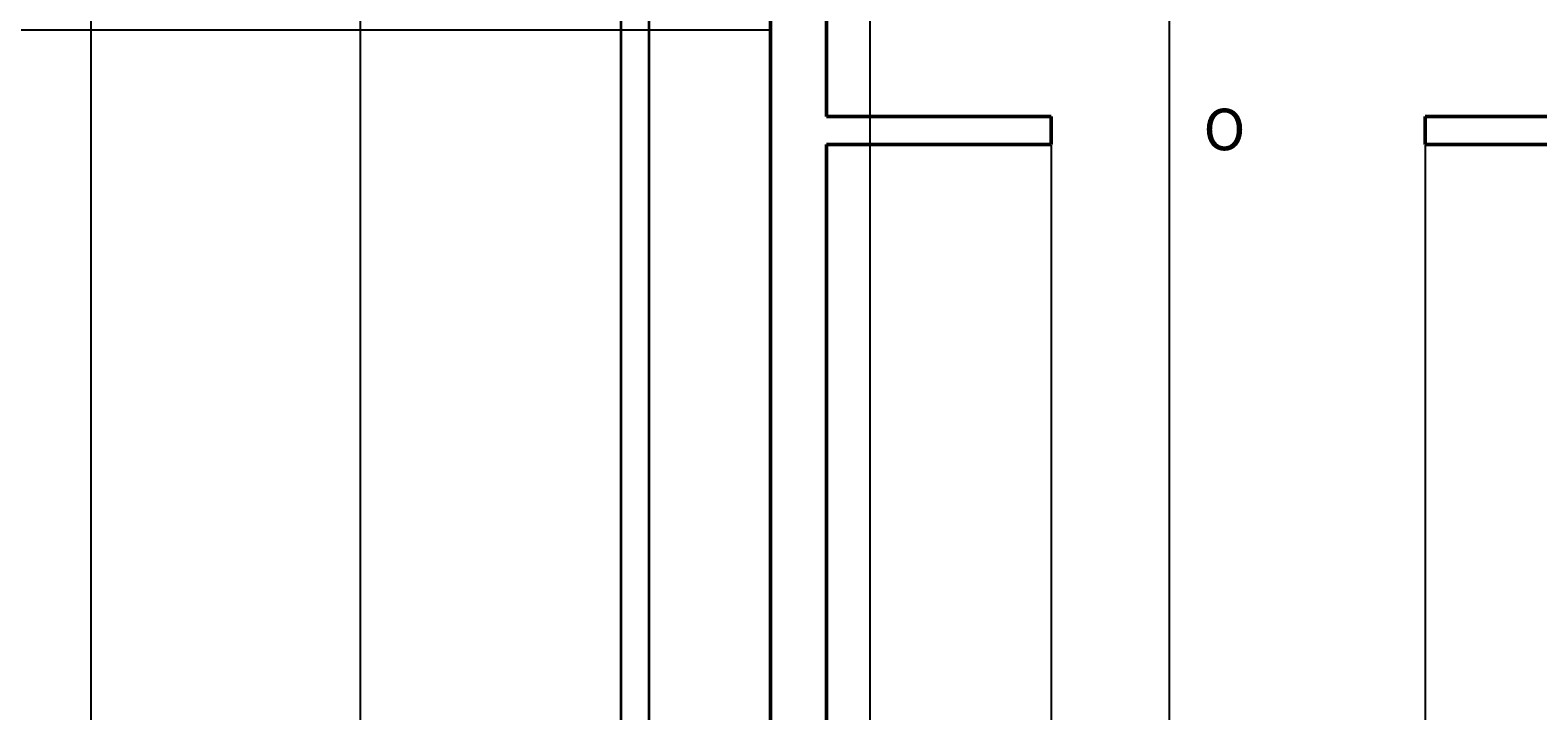
# Model space of a CAD drawing. Units: inches. Extents: x 338 to 1188, y -996 to 127.
# Tile 6 of 15: x 478 to 720, y -240 to -131. Entities that reach past the tile are written whole.
import ezdxf

# ---------------------------------------------------------------- set-up
doc = ezdxf.new("R2010")
doc.units = ezdxf.units.IN
doc.header["$MEASUREMENT"] = 0
for name, color, linetype, lineweight in [('A-ANNO-DIMS', 5, 'Continuous', 18), ('A-ANNO-TEXT', 7, 'Continuous', 18), ('C-PROP', 1, 'Continuous', 35), ('wall', 1, 'Continuous', 50)]:
    doc.layers.add(name, color=color, linetype=linetype, lineweight=lineweight)
doc.styles.get("Standard").update_dxf_attribs({"font": 'arial.ttf'})
doc.dimstyles.get("Standard").update_dxf_attribs({"dimtxt": 0.18, "dimasz": 0.18, "dimexe": 0.18, "dimexo": 0.0625, "dimgap": 0.09, "dimtad": 0, "dimtih": 1, "dimtoh": 1, "dimdec": 1, "dimzin": 0, "dimdsep": 46, "dimlunit": 4, "dimtxsty": 'Standard', "dimcen": 0.09, "dimadec": 0, "dimazin": 0, "dimtfac": 1, "dimtdec": 1, "dimtofl": 0, "dimtmove": 0, "dimatfit": 3, "dimfxl": 1, "dimtolj": 1, "dimtzin": 0, "dimarcsym": 0})

# ---------------------------------------------------------------- blocks, each defined once
blk = doc.blocks.new('_ArchTick')
at = {"color": 0, "linetype": 'ByBlock', "const_width": 0.15}
blk.add_lwpolyline([(-0.5, -0.5), (0.5, 0.5)], dxfattribs=at)
blk = doc.blocks.new('*D6')
at = {"layer": 'A-ANNO-DIMS', "color": 0, "lineweight": -2, "transparency": 16777216}
for p, q in [((531.19, -15.73), (531.19, -304.1)), ((531.19, -615.73), (531.19, -327.37))]:
    blk.add_line(p, q, dxfattribs=at)
at = {"layer": 'Defpoints', "color": 0, "transparency": 16777216}
for p in [(596.96, -15.73), (531.19, -615.73), (596.96, -615.73)]:
    blk.add_point(p, dxfattribs=at)
at = {"layer": 'A-ANNO-DIMS', "color": 0, "lineweight": -2, "transparency": 16777216, "xscale": 10, "yscale": 10, "zscale": 10}
for p, rotation in [((531.19, -15.73), 90), ((531.19, -615.73), 270)]:
    blk.add_blockref('_ArchTick', p, dxfattribs=dict(at, rotation=rotation))
at = {"layer": 'A-ANNO-DIMS', "color": 0, "transparency": 16777216, "insert": (531.19, -315.73), "char_height": 9, "attachment_point": 5, "rotation": 90}
blk.add_mtext("\\A1;50'", dxfattribs=at)
blk = doc.blocks.new('*D7')
at = {"layer": 'A-ANNO-DIMS', "color": 0, "lineweight": -2, "transparency": 16777216}
for p, q in [((488.01, 8.27), (488.01, -388.07)), ((488.01, -807.73), (488.01, -411.39))]:
    blk.add_line(p, q, dxfattribs=at)
at = {"layer": 'Defpoints', "color": 0, "transparency": 16777216}
for p in [(572.96, 8.27), (488.01, -807.73), (572.96, -807.73)]:
    blk.add_point(p, dxfattribs=at)
at = {"layer": 'A-ANNO-DIMS', "color": 0, "lineweight": -2, "transparency": 16777216, "xscale": 10, "yscale": 10, "zscale": 10}
for p, rotation in [((488.01, 8.27), 90), ((488.01, -807.73), 270)]:
    blk.add_blockref('_ArchTick', p, dxfattribs=dict(at, rotation=rotation))
at = {"layer": 'A-ANNO-DIMS', "color": 0, "transparency": 16777216, "insert": (488.01, -399.73), "char_height": 9, "attachment_point": 5, "rotation": 90}
blk.add_mtext("\\A1;68'", dxfattribs=at)
blk = doc.blocks.new('*D31')
at = {"layer": 'A-ANNO-DIMS', "color": 0, "lineweight": -2, "transparency": 16777216}
for p, q in [((641.96, -149.3), (641.96, -968.86)), ((701.96, -149.3), (701.96, -968.86)), ((642.14, -968.68), (671.63, -968.68)), ((701.78, -968.68), (672.29, -968.68))]:
    blk.add_line(p, q, dxfattribs=at)
at = {"layer": 'A-ANNO-DIMS', "color": 0, "transparency": 16777216}
for points in [[(642.14, -968.65), (642.14, -968.71), (641.96, -968.68)], [(701.78, -968.65), (701.78, -968.71), (701.96, -968.68)]]:
    blk.add_solid(points, dxfattribs=at)
at = {"layer": 'Defpoints', "color": 0, "transparency": 16777216}
for p in [(641.96, -149.23), (701.96, -149.23), (701.96, -968.68)]:
    blk.add_point(p, dxfattribs=at)
at = {"layer": 'A-ANNO-DIMS', "color": 0, "transparency": 16777216, "insert": (671.96, -968.68), "char_height": 0.18, "attachment_point": 5}
blk.add_mtext('\\A1;5\'-0"', dxfattribs=at)
blk = doc.blocks.new('*D34')
at = {"layer": 'A-ANNO-DIMS', "color": 0, "lineweight": -2, "transparency": 16777216}
for p, q in [((612.96, -615.67), (612.96, 67.25)), ((613.14, 67.07), (636.63, 67.07)), ((660.78, 67.07), (637.3, 67.07)), ((660.96, -615.67), (660.96, 67.25))]:
    blk.add_line(p, q, dxfattribs=at)
at = {"layer": 'A-ANNO-DIMS', "color": 0, "transparency": 16777216}
for points in [[(613.14, 67.1), (613.14, 67.04), (612.96, 67.07)], [(660.78, 67.1), (660.78, 67.04), (660.96, 67.07)]]:
    blk.add_solid(points, dxfattribs=at)
at = {"layer": 'Defpoints', "color": 0, "transparency": 16777216}
for p in [(660.96, 67.07), (612.96, -615.73), (660.96, -615.73)]:
    blk.add_point(p, dxfattribs=at)
at = {"layer": 'A-ANNO-DIMS', "color": 0, "transparency": 16777216, "insert": (636.96, 67.07), "char_height": 0.18, "attachment_point": 5}
blk.add_mtext('\\A1;4\'-0"', dxfattribs=at)
blk = doc.blocks.new('*D48')
at = {"layer": 'A-ANNO-DIMS', "color": 0, "lineweight": -2, "transparency": 16777216}
for p, q in [((596.96, -615.67), (596.96, 67.25)), ((597.14, 67.07), (604.64, 67.07)), ((612.78, 67.07), (605.28, 67.07)), ((612.96, -615.67), (612.96, 67.25))]:
    blk.add_line(p, q, dxfattribs=at)
at = {"layer": 'A-ANNO-DIMS', "color": 0, "transparency": 16777216}
for points in [[(597.14, 67.1), (597.14, 67.04), (596.96, 67.07)], [(612.78, 67.1), (612.78, 67.04), (612.96, 67.07)]]:
    blk.add_solid(points, dxfattribs=at)
at = {"layer": 'Defpoints', "color": 0, "transparency": 16777216}
for p in [(612.96, 67.07), (596.96, -615.73), (612.96, -615.73)]:
    blk.add_point(p, dxfattribs=at)
at = {"layer": 'A-ANNO-DIMS', "color": 0, "transparency": 16777216, "insert": (604.96, 67.07), "char_height": 0.18, "attachment_point": 5}
blk.add_mtext('\\A1;1\'-4"', dxfattribs=at)
blk = doc.blocks.new('*D51')
at = {"layer": 'A-ANNO-DIMS', "color": 0, "lineweight": -2, "transparency": 16777216}
for p, q in [((596.9, -130.89), (337.66, -130.89)), ((337.84, -131.07), (337.84, -187.13)), ((337.84, -243.55), (337.84, -187.49)), ((596.9, -243.73), (337.66, -243.73))]:
    blk.add_line(p, q, dxfattribs=at)
at = {"layer": 'A-ANNO-DIMS', "color": 0, "transparency": 16777216}
for points in [[(337.81, -131.07), (337.87, -131.07), (337.84, -130.89)], [(337.81, -243.55), (337.87, -243.55), (337.84, -243.73)]]:
    blk.add_solid(points, dxfattribs=at)
at = {"layer": 'Defpoints', "color": 0, "transparency": 16777216}
for p in [(596.96, -130.89), (337.84, -243.73), (596.96, -243.73)]:
    blk.add_point(p, dxfattribs=at)
at = {"layer": 'A-ANNO-DIMS', "color": 0, "transparency": 16777216, "insert": (337.84, -187.31), "char_height": 0.18, "attachment_point": 5}
blk.add_mtext('\\A1;9\'-5"', dxfattribs=at)

msp = doc.modelspace()

# ---------------------------------------------------------------- linework, layer by layer
at = {"layer": 'C-PROP'}
for p, q in [((572.96, 8.27), (572.96, -807.73)), ((577.46, 3.77), (577.46, -803.23))]:
    msp.add_line(p, q, dxfattribs=at)
at = {"layer": 'wall'}
for p, q in [((596.96, -15.73), (596.96, -615.73)), ((605.96, -24.73), (605.96, -144.73)), ((605.96, -24.73), (605.96, -144.73)), ((641.96, -144.73), (605.96, -144.73)), ((641.96, -144.73), (641.96, -149.23)), ((701.96, -144.73), (701.96, -149.23)), ((737.96, -144.73), (701.96, -144.73)), ((605.96, -149.23), (605.96, -606.73)), ((641.96, -149.23), (605.96, -149.23)), ((847.46, -149.23), (701.96, -149.23))]:
    msp.add_line(p, q, dxfattribs=at)

# ---------------------------------------------------------------- texts
at = {"layer": 'A-ANNO-TEXT'}
msp.add_text('O', height=6.65, dxfattribs=at).set_placement((666.4, -150.12))

# ---------------------------------------------------------------- dimensions: what is measured, and where the dimension line sits
at = {"layer": 'A-ANNO-DIMS'}
for base, p1, p2, picture, middle in [((612.96, 67.07), (596.96, -615.73), (612.96, -615.73), '*D48', (604.96, 67.07)), ((660.96, 67.07), (612.96, -615.73), (660.96, -615.73), '*D34', (636.96, 67.07)), ((701.96, -968.68), (641.96, -149.23), (701.96, -149.23), '*D31', (671.96, -968.68))]:
    dim = msp.add_linear_dim(base=base, p1=p1, p2=p2, dimstyle='Standard', override={"dimdec": 1, "dimlfac": 1, "dimrnd": 0, "dimzin": 1, "dimdsep": 46, "dimlunit": 4, "dimfrac": 2}, dxfattribs=at)
    dim.commit()
    dim.dimension.update_dxf_attribs({"geometry": picture, "text_midpoint": middle})
for base, p1, p2, override, picture, middle in [((488.01, -807.73), (572.96, 8.27), (572.96, -807.73), {"dimtxt": 9, "dimasz": 10, "dimgap": 4, "dimtad": 0, "dimtih": 0, "dimblk1": 'ArchTick', "dimblk2": 'ArchTick', "dimsah": 1, "dimse1": 1, "dimse2": 1, "dimclrd": 0, "dimclre": 0, "dimclrt": 0}, '*D7', (488.01, -399.73)), ((531.19, -615.73), (596.96, -15.73), (596.96, -615.73), {"dimtxt": 9, "dimasz": 10, "dimgap": 4, "dimtih": 0, "dimblk1": 'ArchTick', "dimblk2": 'ArchTick', "dimsah": 1, "dimse1": 1, "dimse2": 1, "dimclrd": 0, "dimclre": 0, "dimclrt": 0}, '*D6', (531.19, -315.73)), ((337.84, -243.73), (596.96, -130.89), (596.96, -243.73), {"dimdec": 1, "dimlfac": 1, "dimrnd": 0, "dimzin": 1, "dimdsep": 46, "dimlunit": 4, "dimfrac": 2}, '*D51', (337.84, -187.31))]:
    dim = msp.add_linear_dim(base=base, p1=p1, p2=p2, angle=90, dimstyle='Standard', override=override, dxfattribs=at)
    dim.commit()
    dim.dimension.update_dxf_attribs({"geometry": picture, "text_midpoint": middle})

doc.saveas('drawing.dxf')
